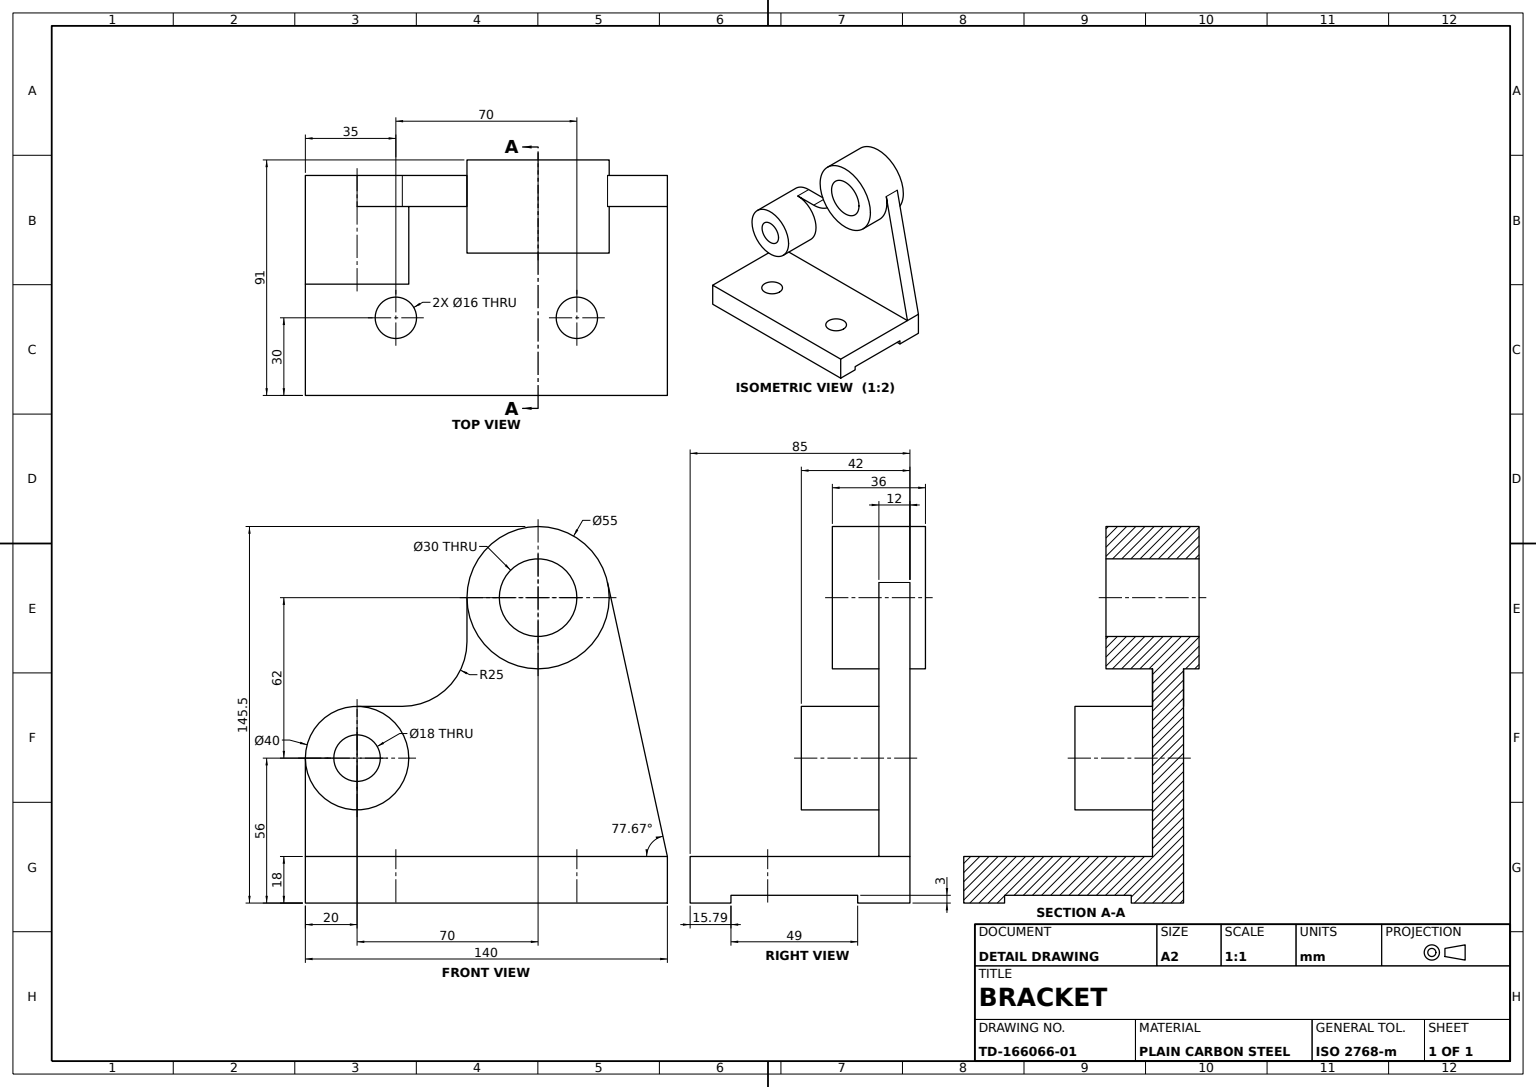
from build123d import *

# Parameters (mm, degrees)
BRACKET_PROFILE_SKETCH_R   = 15
BRACKET_PROFILE_SKETCH_R_2 = 9
BRACKET_BODY_DEPTH         = 85
GUSSET_TRIM_SKETCH_W       = 152.495630812
GUSSET_TRIM_SKETCH_H       = 155.202581702
GUSSET_TRIM_CUT_DEPTH      = 73
BASE_GROOVE_SKETCH_W       = 49
BASE_GROOVE_SKETCH_H       = 3
BASE_GROOVE_DEPTH          = 202.86381548
PIVOT_BOSSES_SKETCH_R      = 15
PIVOT_BOSS_36MM_DEPTH      = 18
SKETCH13_3_R               = 9
PIVOT_BOSS_30MM_DEPTH      = 30
MOUNTING_HOLES_SKETCH_R    = 8
BASE_MOUNTING_HOLES_DEPTH  = 30


with BuildPart() as part:
    # Bracket Profile Sketch → Bracket Body (new body)
    with BuildSketch(Plane.XY):
        with BuildLine():
            Line((-90, -62), (-90, -118))
            Line((-90, -118), (50, -118))
            Line((50, -118), (50, -100))
            Line((50, -100), (26.866088482, 5.870544241))
            ThreePointArc((26.866088482, 5.870544241), (-2.952335241, 27.341062829), (-27.5, 0))
            Line((-27.5, 0), (-27.5, -17))
            ThreePointArc((-27.5, -17), (-34.82233047, -34.67766953), (-52.5, -42))
            Line((-52.5, -42), (-70, -42))
            ThreePointArc((-70, -42), (-84.142135624, -47.857864376), (-90, -62))
        make_face()
        Circle(BRACKET_PROFILE_SKETCH_R, mode=Mode.SUBTRACT)
        with Locations((-70, -62)):
            Circle(BRACKET_PROFILE_SKETCH_R_2, mode=Mode.SUBTRACT)
    extrude(amount=BRACKET_BODY_DEPTH)

    # Gusset Trim Sketch → Gusset Trim Cut (cut)
    with BuildSketch(Plane.XY.offset(85)):
        with Locations((-26.247815406, -22.398709149)):
            Rectangle(GUSSET_TRIM_SKETCH_W, GUSSET_TRIM_SKETCH_H)
    extrude(amount=-GUSSET_TRIM_CUT_DEPTH, mode=Mode.SUBTRACT)

    # Base Groove Sketch → Base Groove (cut, through all)
    with BuildSketch(Plane.ZY.offset(90)):
        with Locations((44.711476451, -116.5)):
            Rectangle(BASE_GROOVE_SKETCH_W, BASE_GROOVE_SKETCH_H)
    extrude(amount=-BASE_GROOVE_DEPTH, mode=Mode.SUBTRACT)

    # Pivot Bosses Sketch → Pivot Boss 36mm (add, symmetric)
    with BuildSketch(Plane.XY.offset(12)):
        with BuildLine():
            ThreePointArc((-27.5, 0), (0, -27.5), (27.5, 0))
            ThreePointArc((27.5, 0), (27.341062829, 2.952335241), (26.866088482, 5.870544241))
            ThreePointArc((26.866088482, 5.870544241), (-2.952335241, 27.341062829), (-27.5, 0))
        make_face()
        Circle(PIVOT_BOSSES_SKETCH_R, mode=Mode.SUBTRACT)
    extrude(amount=PIVOT_BOSS_36MM_DEPTH, both=True)

    # Sketch13_3 → Pivot Boss 30mm (add)
    with BuildSketch(Plane.XY.offset(12)):
        with BuildLine():
            ThreePointArc((-90, -62), (-70, -82), (-50, -62))
            ThreePointArc((-50, -62), (-55.857864376, -47.857864376), (-70, -42))
            ThreePointArc((-70, -42), (-84.142135624, -47.857864376), (-90, -62))
        make_face()
        with Locations((-70, -62)):
            Circle(SKETCH13_3_R, mode=Mode.SUBTRACT)
    extrude(amount=PIVOT_BOSS_30MM_DEPTH)

    # Mounting Holes Sketch → Base Mounting Holes (cut)
    with BuildSketch(Plane(origin=(0, -100, 0), x_dir=(1, 0, 0), z_dir=(0, 1, 0))):
        with Locations(Location((-55, -55, 0), (0, 0, 180))):
            Circle(MOUNTING_HOLES_SKETCH_R)
        with Locations(Location((15, -55, 0), (0, 0, 180))):
            Circle(MOUNTING_HOLES_SKETCH_R)
    extrude(amount=-BASE_MOUNTING_HOLES_DEPTH, mode=Mode.SUBTRACT)


solid = part.part
